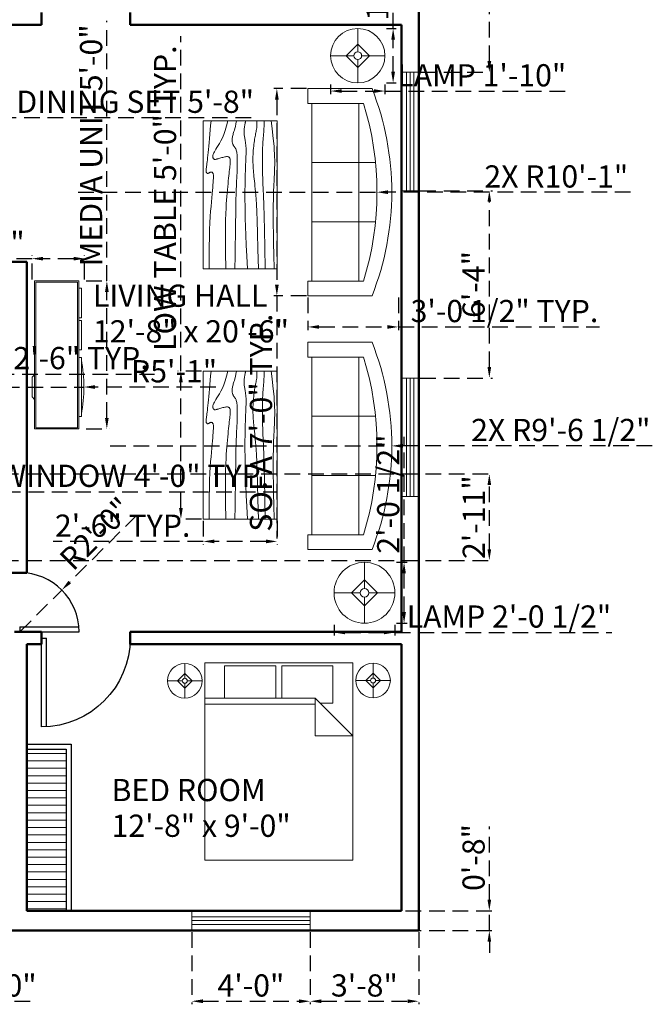
# Model space of a CAD drawing. Units: inches. Extents: x 3209 to 7144, y 1281 to 3076.
# Tile 3 of 5: x 3474 to 3731, y 1281 to 1680. Entities that reach past the tile are written whole.
import ezdxf

# ---------------------------------------------------------------- set-up
doc = ezdxf.new("R2010")
doc.units = ezdxf.units.IN
doc.linetypes.add('HIDDEN', pattern=[9.525, 6.35, -3.175])
for name, color, linetype, lineweight in [('A-ANNO-DIMS', 244, 'HIDDEN', 18), ('A-AREA-IDEN', 7, 'Continuous', 25), ('A-DOOR', 4, 'Continuous', 25), ('A-FLOR-CASE', 8, 'Continuous', 25), ('A-FLOR-CASE-PATT', 252, 'Continuous', 13), ('A-FURN', 8, 'Continuous', 18), ('A-GLAZ', 4, 'Continuous', 18), ('A-WALL', 7, 'Continuous', 50)]:
    doc.layers.add(name, color=color, linetype=linetype, lineweight=lineweight)
doc.styles.get("Standard").update_dxf_attribs({"font": 'arial.ttf'})
doc.dimstyles.new('ISO-25', dxfattribs={"dimtxt": 9, "dimasz": 4.5, "dimexe": 1.25, "dimexo": 0.625, "dimtad": 1, "dimdec": 0, "dimlunit": 3, "dimtxsty": 'Standard', "dimcen": 2.5, "dimadec": 0, "dimazin": 0, "dimtfac": 1, "dimtdec": 0, "dimtmove": 0, "dimatfit": 3, "dimfxl": 1, "dimarcsym": 0})

# ---------------------------------------------------------------- blocks, each defined once
blk = doc.blocks.new('Entertainment Center')
for p, q in [((-4, 0), (-5, -1)), ((4, 0), (-4, 0)), ((5, -1), (4, 0)), ((-17, -19), (-17, -1)), ((-17, -1), (43, -1)), ((-16.5, -18.5), (-16.5, -1.5)), ((-16.5, -1.5), (42.5, -1.5)), ((42.5, -1.5), (42.5, -18.5)), ((43, -1), (43, -19)), ((43, -19), (-17, -19)), ((42.5, -18.5), (-16.5, -18.5)), ((-12, -20), (-12, -19)), ((12, -19), (12, -20)), ((15, -20), (15, -19)), ((27, -19), (27, -20)), ((28, -20), (28, -19)), ((40, -19), (40, -20)), ((12, -20), (-12, -20)), ((27, -20), (15, -20)), ((40, -20), (28, -20))]:
    blk.add_line(p, q)
blk.add_arc((0, 40), 61, 259.6111, 280.3889)
blk = doc.blocks.new('Sofa - Roundback 7 ft.')
for p, q in [((-12.00002, -32.4421), (-12.00003, -6.5971)), ((11.99997, -32.4421), (11.99998, -6.5971)), ((-36.000027, -34), (-36.000027, -11.4696)), ((35.99998, -34), (35.99998, -11.4696)), ((-35.999844, -13.3819), (35.9998, -13.3819)), ((-36.000027, -32.4421), (35.99998, -32.4421))]:
    blk.add_line(p, q)
for points in [[(-36.000027, -34), (-42.000027, -34), (-42.000027, -8)], [(41.99998, -8), (41.99998, -34), (35.99998, -34)]]:
    blk.add_lwpolyline(points)
for centre, radius, start, end in [((0, -114.25), 114.25, 68.43141, 111.5686), ((-0.00001, -127.1968), 121.1968, 72.72033, 107.2797)]:
    blk.add_arc(centre, radius, start, end)
blk = doc.blocks.new('Table - Rectangular Woodgrain 60 x 30 in.')
for p, q in [((0, 0), (0, -30)), ((60, 0), (0, 0)), ((60, -30), (60, 0)), ((0, -30), (60, -30))]:
    blk.add_line(p, q)
for points in [[(0, -2.4), (4.8155, -2.418), (9.0302, -2.4688), (12.709, -2.5477), (15.9167, -2.65), (18.7181, -2.7711), (21.1781, -2.9063), (23.3616, -3.0508), (25.3333, -3.2), (27.1477, -3.3495), (28.8172, -3.4958), (30.3437, -3.636), (31.7291, -3.7667), (32.9756, -3.8849), (34.0849, -3.9875), (35.059, -4.0714), (35.9, -4.1334), (36.6114, -4.1711), (37.2041, -4.1854), (37.6906, -4.1779), (38.0833, -4.15), (38.3948, -4.1034), (38.6375, -4.0396), (38.8239, -3.9602), (38.9666, -3.8667), (39.0764, -3.7608), (39.1573, -3.6448), (39.2116, -3.521), (39.2416, -3.3917), (39.2498, -3.2593), (39.2385, -3.1261), (39.21, -2.9944), (39.1666, -2.8667), (39.111, -2.7447), (39.0468, -2.6281), (38.978, -2.5163), (38.9083, -2.4083), (38.8418, -2.3035), (38.7823, -2.201), (38.7337, -2.1001), (38.7, -2), (38.6844, -1.9003), (38.6875, -1.8021), (38.7094, -1.707), (38.75, -1.6167), (38.8094, -1.5326), (38.8875, -1.4563), (38.9844, -1.3893), (39.1, -1.3333), (39.2351, -1.2896), (39.3937, -1.2583), (39.5804, -1.2396), (39.8, -1.2333), (40.057, -1.2396), (40.3562, -1.2583), (40.7023, -1.2896), (41.1, -1.3333), (41.5547, -1.3895), (42.0755, -1.4573), (42.6721, -1.5361), (43.3542, -1.625), (44.1316, -1.7233), (45.014, -1.8302), (46.0114, -1.9449), (47.1333, -2.0667), (48.3862, -2.1947), (49.7625, -2.3281), (51.2513, -2.4663), (52.8416, -2.6083), (54.5226, -2.7535), (56.2833, -2.9011), (58.1127, -3.0501), (60, -3.2)], [(0, -9.2), (6.5759, -9.0858), (11.9385, -9.0365), (16.2527, -9.0418), (19.6833, -9.0917), (22.3952, -9.1759), (24.5531, -9.2844), (26.322, -9.4069), (27.8666, -9.5333), (29.3241, -9.6553), (30.7203, -9.7719), (32.0532, -9.8837), (33.3208, -9.9917), (34.5213, -10.0965), (35.6526, -10.199), (36.7128, -10.2999), (37.7, -10.4), (38.6129, -10.4996), (39.4531, -10.5969), (40.223, -10.6895), (40.925, -10.775), (41.5613, -10.8512), (42.1344, -10.9156), (42.6465, -10.966), (43.1, -11), (43.4976, -11.0158), (43.8437, -11.0136), (44.143, -10.9942), (44.4, -10.9583), (44.6195, -10.9069), (44.8062, -10.8406), (44.9648, -10.7603), (45.1, -10.6667), (45.2155, -10.5598), (45.3114, -10.4365), (45.3871, -10.2929), (45.4416, -10.125), (45.4743, -9.929), (45.4844, -9.7011), (45.4709, -9.4371), (45.4333, -9.1333), (45.3716, -8.7883), (45.2896, -8.4104), (45.1919, -8.0107), (45.0833, -7.6), (44.9685, -7.1893), (44.8521, -6.7896), (44.7388, -6.4117), (44.6333, -6.0667), (44.54, -5.7628), (44.4614, -5.4979), (44.4001, -5.2675), (44.3583, -5.0667), (44.3384, -4.8909), (44.3427, -4.7354), (44.3736, -4.5956), (44.4333, -4.4667), (44.5236, -4.3453), (44.6427, -4.2333), (44.7884, -4.1339), (44.9583, -4.05), (45.1501, -3.9849), (45.3614, -3.9417), (45.59, -3.9234), (45.8333, -3.9333), (46.0915, -3.9749), (46.3734, -4.0531), (46.6906, -4.1736), (47.0542, -4.3417), (47.4756, -4.5629), (47.9661, -4.8427), (48.5372, -5.1866), (49.2, -5.6), (49.9676, -6.0844), (50.8594, -6.625), (51.8965, -7.2031), (53.1, -7.8), (54.491, -8.3969), (56.0906, -8.975), (57.9199, -9.5156), (60, -10)], [(0, -12.8), (5.1847, -12.9322), (9.6213, -13.0323), (13.3963, -13.1059), (16.5958, -13.1583), (19.3063, -13.1952), (21.614, -13.2219), (23.6054, -13.2439), (25.3666, -13.2667), (26.9728, -13.2947), (28.4531, -13.3281), (29.8256, -13.3663), (31.1083, -13.4083), (32.3191, -13.4535), (33.476, -13.501), (34.597, -13.5501), (35.7, -13.6), (36.7984, -13.6497), (37.8875, -13.6979), (38.9578, -13.743), (40, -13.7833), (41.0047, -13.8174), (41.9625, -13.8438), (42.864, -13.8607), (43.7, -13.8667), (44.4631, -13.8604), (45.1552, -13.8417), (45.7801, -13.8104), (46.3416, -13.7667), (46.8439, -13.7104), (47.2906, -13.6417), (47.6858, -13.5604), (48.0333, -13.4667), (48.3375, -13.3608), (48.6042, -13.2448), (48.8396, -13.121), (49.05, -12.9917), (49.2417, -12.8593), (49.4208, -12.7261), (49.5937, -12.5944), (49.7667, -12.4667), (49.9452, -12.3451), (50.1323, -12.2313), (50.3303, -12.1268), (50.5416, -12.0333), (50.7686, -11.9524), (51.0135, -11.8854), (51.2788, -11.8341), (51.5666, -11.8), (51.8785, -11.7843), (52.2116, -11.7865), (52.562, -11.8059), (52.926, -11.8417), (53.2998, -11.8931), (53.6795, -11.9594), (54.0614, -12.0397), (54.4416, -12.1333), (54.8223, -12.2401), (55.2293, -12.3625), (55.6942, -12.5037), (56.2489, -12.6667), (56.9251, -12.8547), (57.7545, -13.0708), (58.7689, -13.3182), (60, -13.6)], [(0, -18), (5.124, -17.7273), (9.6609, -17.5057), (13.6705, -17.3303), (17.2125, -17.1958), (20.3467, -17.0973), (23.1328, -17.0297), (25.6307, -16.9878), (27.9, -16.9667), (29.9928, -16.9617), (31.9302, -16.9703), (33.7254, -16.9907), (35.3917, -17.0208), (36.9423, -17.0588), (38.3906, -17.1026), (39.7499, -17.1503), (41.0333, -17.2), (42.2519, -17.2496), (43.4073, -17.2969), (44.4986, -17.3395), (45.525, -17.375), (46.4858, -17.4012), (47.3802, -17.4156), (48.2074, -17.416), (48.9667, -17.4), (49.6583, -17.3662), (50.2872, -17.3167), (50.8595, -17.2547), (51.3812, -17.1833), (51.8584, -17.1057), (52.2971, -17.025), (52.7034, -16.9443), (53.0833, -16.8667), (53.443, -16.7951), (53.789, -16.7313), (54.128, -16.6768), (54.4666, -16.6334), (54.8115, -16.6024), (55.1693, -16.5854), (55.5465, -16.5841), (55.95, -16.6), (56.3828, -16.6337), (56.8346, -16.6823), (57.2915, -16.7418), (57.7396, -16.8084), (58.165, -16.878), (58.5539, -16.9469), (58.8924, -17.0111), (59.1666, -17.0667), (59.3679, -17.1107), (59.5078, -17.1438), (59.6032, -17.1675), (59.6708, -17.1833), (59.7275, -17.193), (59.7901, -17.1979), (59.8753, -17.1998), (60, -17.2)], [(0, -22.4), (8.0098, -22.2501), (14.4094, -22.1011), (19.4168, -21.9535), (23.25, -21.8083), (26.1269, -21.6663), (28.2656, -21.5281), (29.884, -21.3947), (31.2, -21.2667), (32.3967, -21.1448), (33.5172, -21.0292), (34.5697, -20.9198), (35.5625, -20.8167), (36.5037, -20.7198), (37.4015, -20.6292), (38.2642, -20.5448), (39.1, -20.4667), (39.9164, -20.3951), (40.7187, -20.3313), (41.5117, -20.2768), (42.3, -20.2333), (43.0883, -20.2024), (43.8812, -20.1854), (44.6836, -20.1841), (45.5, -20.2), (46.3328, -20.234), (47.1747, -20.2844), (48.0163, -20.3488), (48.8479, -20.425), (49.66, -20.5106), (50.4429, -20.6031), (51.1872, -20.7004), (51.8833, -20.8), (52.5246, -20.8999), (53.1166, -20.9995), (53.6681, -21.0983), (54.1875, -21.1958), (54.6834, -21.2919), (55.1646, -21.3859), (55.6394, -21.4777), (56.1167, -21.5667), (56.6028, -21.6515), (57.0961, -21.7266), (57.5929, -21.7852), (58.0896, -21.8208), (58.5823, -21.8268), (59.0674, -21.7964), (59.5412, -21.723), (60, -21.6)], [(0, -25.2), (8.6355, -25.0504), (15.7026, -24.9031), (21.4049, -24.7606), (25.9458, -24.625), (29.529, -24.4988), (32.3578, -24.3844), (34.6359, -24.284), (36.5667, -24.2), (38.3213, -24.1341), (39.9417, -24.0854), (41.437, -24.0523), (42.8167, -24.0333), (44.0901, -24.0268), (45.2667, -24.0313), (46.3557, -24.0451), (47.3667, -24.0667), (48.309, -24.0947), (49.1928, -24.1287), (50.0284, -24.168), (50.826, -24.2125), (51.5959, -24.2617), (52.3483, -24.3151), (53.0935, -24.3725), (53.8417, -24.4334), (54.6009, -24.497), (55.3699, -24.561), (56.1454, -24.6226), (56.9239, -24.6792), (57.7021, -24.7279), (58.4764, -24.7662), (59.2435, -24.7911), (60, -24.8)], [(0, -28.8), (5.6867, -28.6681), (10.45, -28.5698), (14.407, -28.5012), (17.675, -28.4584), (20.3711, -28.4374), (22.6125, -28.4344), (24.5164, -28.4455), (26.2, -28.4667), (27.762, -28.4947), (29.2276, -28.5281), (30.6033, -28.5663), (31.8958, -28.6084), (33.1118, -28.6535), (34.2578, -28.7011), (35.3405, -28.7501), (36.3666, -28.8), (37.3443, -28.8497), (38.288, -28.8974), (39.2137, -28.9412), (40.1375, -28.9792), (41.0753, -29.0093), (42.0432, -29.0297), (43.0572, -29.0384), (44.1333, -29.0333), (45.2936, -29.0114), (46.5843, -28.9641), (48.0579, -28.8816), (49.7666, -28.7542), (51.7629, -28.5721), (54.0989, -28.3255), (56.8272, -28.0048), (60, -27.6)]]:
    blk.add_lwpolyline(points)
blk = doc.blocks.new('Bed - Queen')
for p, q in [((0, -80.00003), (0, 0)), ((0, 0), (59.99999, 0)), ((59.99999, 0), (59.99999, -80.00003)), ((7.99999, -1.2), (28.79998, -1.2)), ((7.99999, -14.4), (7.99999, -1.2)), ((28.79998, -1.2), (28.79998, -14.4)), ((31.19999, -1.2), (51.99999, -1.2)), ((31.19999, -14.4), (31.19999, -1.2)), ((51.99999, -1.2), (51.99999, -16.4)), ((0, -14.4), (44.8, -14.4)), ((59.99999, -29.6), (44.8, -14.4)), ((44.8, -14.4), (44.8, -29.6)), ((44.8, -16.8), (0, -16.8)), ((51.99999, -16.4), (46.79936, -16.4)), ((44.8, -29.6), (59.99999, -29.6)), ((59.99999, -80.00003), (0, -80.00003))]:
    blk.add_line(p, q)
blk = doc.blocks.new('Lamp - Table')
for p, q in [((0, 7), (0, 1)), ((0, 3), (-3, 0)), ((3, 0), (0, 3)), ((-1, 0), (-7, 0)), ((-3, 0), (0, -3)), ((0, -3), (3, 0)), ((1, 0), (7, 0)), ((0, -1), (0, -7))]:
    blk.add_line(p, q)
for radius in [7, 1]:
    blk.add_circle((0, 0), radius)
blk = doc.blocks.new('DOOR-SWING-36IN')
for p, q in [((0, 36), (0, 0)), ((2, 36), (2, 0)), ((0, 0), (2, 0))]:
    blk.add_line(p, q)
blk.add_arc((0, 0), 36, 0, 90)
blk = doc.blocks.new('WINDOW-48IN-WALL7')
for p, q in [((0, 48), (7, 48)), ((2, 48), (2, 0)), ((3.5, 48), (3.5, 0)), ((5, 48), (5, 0)), ((0, 0), (7, 0))]:
    blk.add_line(p, q)
blk = doc.blocks.new('CASEWORK-BEDROOM-SURROUND')
for p, q in [((0, 67.48), (18, 67.48)), ((0, 65.48), (16, 65.48)), ((16, 65.48), (16, 0)), ((18, 67.48), (18, 0))]:
    blk.add_line(p, q)
blk = doc.blocks.new('*D26')
at = {"layer": 'A-ANNO-DIMS', "color": 0, "lineweight": -2, "transparency": 16777216}
for p, q in [((3600.19, 1654.1), (3600.19, 1650.17)), ((3622.25, 1654.1), (3622.25, 1650.17)), ((3604.69, 1651.42), (3617.75, 1651.42)), ((3622.25, 1651.42), (3696.25, 1651.42))]:
    blk.add_line(p, q, dxfattribs=at)
at = {"layer": 'A-ANNO-DIMS', "color": 0, "transparency": 16777216}
for points in [[(3604.69, 1652.17), (3604.69, 1650.67), (3600.19, 1651.42)], [(3617.75, 1652.17), (3617.75, 1650.67), (3622.25, 1651.42)]]:
    blk.add_solid(points, dxfattribs=at)
at = {"layer": 'Defpoints', "color": 0, "transparency": 16777216}
for p in [(3600.19, 1654.72), (3622.25, 1654.72), (3622.25, 1651.42)]:
    blk.add_point(p, dxfattribs=at)
at = {"layer": 'A-ANNO-DIMS', "color": 0, "transparency": 16777216, "insert": (3661.5, 1656.64), "char_height": 9, "attachment_point": 5}
blk.add_mtext('LAMP 1\'-10"', dxfattribs=at)
blk = doc.blocks.new('*D27')
at = {"layer": 'A-ANNO-DIMS', "color": 0, "lineweight": -2, "transparency": 16777216}
for p, q in [((3625.56, 1676.78), (3625.56, 1712.6)), ((3622.87, 1676.78), (3626.81, 1676.78)), ((3625.56, 1659.22), (3625.56, 1672.28)), ((3622.87, 1654.72), (3626.81, 1654.72))]:
    blk.add_line(p, q, dxfattribs=at)
at = {"layer": 'A-ANNO-DIMS', "color": 0, "transparency": 16777216}
for points in [[(3624.81, 1672.28), (3626.31, 1672.28), (3625.56, 1676.78)], [(3624.81, 1659.22), (3626.31, 1659.22), (3625.56, 1654.72)]]:
    blk.add_solid(points, dxfattribs=at)
at = {"layer": 'Defpoints', "color": 0, "transparency": 16777216}
for p in [(3622.25, 1676.78), (3625.56, 1676.78), (3622.25, 1654.72)]:
    blk.add_point(p, dxfattribs=at)
at = {"layer": 'A-ANNO-DIMS', "color": 0, "transparency": 16777216, "insert": (3620.34, 1696.94), "char_height": 9, "attachment_point": 5, "rotation": 90}
blk.add_mtext('1\'-10"', dxfattribs=at)
blk = doc.blocks.new('*D28')
at = {"layer": 'A-ANNO-DIMS', "color": 0, "lineweight": -2, "transparency": 16777216}
for p, q in [((3601.6, 1435.14), (3601.6, 1430.81)), ((3626.3, 1435.14), (3626.3, 1430.81)), ((3606.1, 1432.06), (3621.8, 1432.06)), ((3626.3, 1432.06), (3714.28, 1432.06))]:
    blk.add_line(p, q, dxfattribs=at)
at = {"layer": 'A-ANNO-DIMS', "color": 0, "transparency": 16777216}
for points in [[(3606.1, 1432.81), (3606.1, 1431.31), (3601.6, 1432.06)], [(3621.8, 1432.81), (3621.8, 1431.31), (3626.3, 1432.06)]]:
    blk.add_solid(points, dxfattribs=at)
at = {"layer": 'Defpoints', "color": 0, "transparency": 16777216}
for p in [(3601.6, 1435.77), (3626.3, 1435.77), (3626.3, 1432.06)]:
    blk.add_point(p, dxfattribs=at)
at = {"layer": 'A-ANNO-DIMS', "color": 0, "transparency": 16777216, "insert": (3672.54, 1437.34), "char_height": 9, "attachment_point": 5}
blk.add_mtext('LAMP 2\'-0 1/2"', dxfattribs=at)
blk = doc.blocks.new('*D29')
at = {"layer": 'A-ANNO-DIMS', "color": 0, "lineweight": -2, "transparency": 16777216}
for p, q in [((3630, 1460.47), (3630, 1511.27)), ((3626.93, 1460.47), (3631.25, 1460.47)), ((3630, 1440.27), (3630, 1455.97)), ((3626.93, 1435.77), (3631.25, 1435.77))]:
    blk.add_line(p, q, dxfattribs=at)
at = {"layer": 'A-ANNO-DIMS', "color": 0, "transparency": 16777216}
for points in [[(3629.25, 1455.97), (3630.75, 1455.97), (3630, 1460.47)], [(3629.25, 1440.27), (3630.75, 1440.27), (3630, 1435.77)]]:
    blk.add_solid(points, dxfattribs=at)
at = {"layer": 'Defpoints', "color": 0, "transparency": 16777216}
for p in [(3626.3, 1460.47), (3630, 1460.47), (3626.3, 1435.77)]:
    blk.add_point(p, dxfattribs=at)
at = {"layer": 'A-ANNO-DIMS', "color": 0, "transparency": 16777216, "insert": (3624.73, 1488.12), "char_height": 9, "attachment_point": 5, "rotation": 90}
blk.add_mtext('2\'-0 1/2"', dxfattribs=at)
blk = doc.blocks.new('*D34')
at = {"layer": 'A-ANNO-DIMS', "color": 0, "lineweight": -2, "transparency": 16777216}
for p, q in [((3539.5, 1537.94), (3539.5, 1673.6)), ((3547.87, 1537.94), (3538.25, 1537.94)), ((3539.5, 1482.44), (3539.5, 1533.44)), ((3547.87, 1477.94), (3538.25, 1477.94))]:
    blk.add_line(p, q, dxfattribs=at)
at = {"layer": 'A-ANNO-DIMS', "color": 0, "transparency": 16777216}
for points in [[(3538.75, 1533.44), (3540.25, 1533.44), (3539.5, 1537.94)], [(3538.75, 1482.44), (3540.25, 1482.44), (3539.5, 1477.94)]]:
    blk.add_solid(points, dxfattribs=at)
at = {"layer": 'Defpoints', "color": 0, "transparency": 16777216}
for p in [(3539.5, 1537.94), (3548.5, 1537.94), (3548.5, 1477.94)]:
    blk.add_point(p, dxfattribs=at)
at = {"layer": 'A-ANNO-DIMS', "color": 0, "transparency": 16777216, "insert": (3534.22, 1608.02), "char_height": 9, "attachment_point": 5, "rotation": 90}
blk.add_mtext('LOW TABLE 5\'-0" TYP.', dxfattribs=at)
blk = doc.blocks.new('*D35')
at = {"layer": 'A-ANNO-DIMS', "color": 0, "lineweight": -2, "transparency": 16777216}
for p, q in [((3548.5, 1477.31), (3548.5, 1467.69)), ((3578.5, 1477.31), (3578.5, 1467.69)), ((3548.5, 1468.94), (3487.74, 1468.94)), ((3574, 1468.94), (3553, 1468.94))]:
    blk.add_line(p, q, dxfattribs=at)
at = {"layer": 'A-ANNO-DIMS', "color": 0, "transparency": 16777216}
for points in [[(3553, 1469.69), (3553, 1468.19), (3548.5, 1468.94)], [(3574, 1469.69), (3574, 1468.19), (3578.5, 1468.94)]]:
    blk.add_solid(points, dxfattribs=at)
at = {"layer": 'Defpoints', "color": 0, "transparency": 16777216}
for p in [(3548.5, 1477.94), (3578.5, 1477.94), (3548.5, 1468.94)]:
    blk.add_point(p, dxfattribs=at)
at = {"layer": 'A-ANNO-DIMS', "color": 0, "transparency": 16777216, "insert": (3515.87, 1474.16), "char_height": 9, "attachment_point": 5}
blk.add_mtext('2\'-6" TYP.', dxfattribs=at)
blk = doc.blocks.new('*D40')
at = {"layer": 'A-ANNO-DIMS', "color": 0, "lineweight": -2, "transparency": 16777216}
for p, q in [((3590.38, 1652.44), (3577.16, 1652.44)), ((3578.41, 1647.94), (3578.41, 1572.94)), ((3590.38, 1568.44), (3577.16, 1568.44)), ((3578.41, 1568.44), (3578.41, 1470.15))]:
    blk.add_line(p, q, dxfattribs=at)
at = {"layer": 'A-ANNO-DIMS', "color": 0, "transparency": 16777216}
for points in [[(3577.66, 1647.94), (3579.16, 1647.94), (3578.41, 1652.44)], [(3577.66, 1572.94), (3579.16, 1572.94), (3578.41, 1568.44)]]:
    blk.add_solid(points, dxfattribs=at)
at = {"layer": 'Defpoints', "color": 0, "transparency": 16777216}
for p in [(3591.01, 1652.44), (3578.41, 1568.44), (3591.01, 1568.44)]:
    blk.add_point(p, dxfattribs=at)
at = {"layer": 'A-ANNO-DIMS', "color": 0, "transparency": 16777216, "insert": (3573.13, 1517.05), "char_height": 9, "attachment_point": 5, "rotation": 90}
blk.add_mtext('SOFA 7\'-0" TYP.', dxfattribs=at)
blk = doc.blocks.new('*D41')
at = {"layer": 'A-ANNO-DIMS', "color": 0, "lineweight": -2, "transparency": 16777216}
for p, q in [((3591.01, 1567.82), (3591.01, 1554.59)), ((3627.68, 1567.82), (3627.68, 1554.59)), ((3595.51, 1555.84), (3623.18, 1555.84)), ((3627.68, 1555.84), (3709.25, 1555.84))]:
    blk.add_line(p, q, dxfattribs=at)
at = {"layer": 'A-ANNO-DIMS', "color": 0, "transparency": 16777216}
for points in [[(3595.51, 1556.59), (3595.51, 1555.09), (3591.01, 1555.84)], [(3623.18, 1556.59), (3623.18, 1555.09), (3627.68, 1555.84)]]:
    blk.add_solid(points, dxfattribs=at)
at = {"layer": 'Defpoints', "color": 0, "transparency": 16777216}
for p in [(3591.01, 1568.44), (3627.68, 1568.44), (3627.68, 1555.84)]:
    blk.add_point(p, dxfattribs=at)
at = {"layer": 'A-ANNO-DIMS', "color": 0, "transparency": 16777216, "insert": (3670.71, 1561.12), "char_height": 9, "attachment_point": 5}
blk.add_mtext('3\'-0 1/2" TYP.', dxfattribs=at)
blk = doc.blocks.new('*D42')
at = {"layer": 'A-ANNO-DIMS', "color": 0, "lineweight": -2, "transparency": 16777216}
for p, q in [((3397.44, 1540.64), (3397.44, 1535.52)), ((3427.44, 1540.64), (3427.44, 1535.52)), ((3401.94, 1536.77), (3422.94, 1536.77)), ((3427.44, 1536.77), (3528.81, 1536.77))]:
    blk.add_line(p, q, dxfattribs=at)
at = {"layer": 'A-ANNO-DIMS', "color": 0, "transparency": 16777216}
for points in [[(3401.94, 1537.52), (3401.94, 1536.02), (3397.44, 1536.77)], [(3422.94, 1537.52), (3422.94, 1536.02), (3427.44, 1536.77)]]:
    blk.add_solid(points, dxfattribs=at)
at = {"layer": 'Defpoints', "color": 0, "transparency": 16777216}
for p in [(3397.44, 1541.27), (3427.44, 1541.27), (3427.44, 1536.77)]:
    blk.add_point(p, dxfattribs=at)
at = {"layer": 'A-ANNO-DIMS', "color": 0, "transparency": 16777216, "insert": (3480.37, 1542.05), "char_height": 9, "attachment_point": 5}
blk.add_mtext('DOOR 2\'-6" TYP.', dxfattribs=at)
blk = doc.blocks.new('*D46')
at = {"layer": 'A-ANNO-DIMS', "color": 0, "lineweight": -2, "transparency": 16777216}
for p, q in [((3410.58, 1495.64), (3410.58, 1487.82)), ((3458.58, 1495.64), (3458.58, 1487.82)), ((3415.08, 1489.07), (3454.08, 1489.07)), ((3458.58, 1489.07), (3578.22, 1489.07))]:
    blk.add_line(p, q, dxfattribs=at)
at = {"layer": 'A-ANNO-DIMS', "color": 0, "transparency": 16777216}
for points in [[(3415.08, 1489.82), (3415.08, 1488.32), (3410.58, 1489.07)], [(3454.08, 1489.82), (3454.08, 1488.32), (3458.58, 1489.07)]]:
    blk.add_solid(points, dxfattribs=at)
at = {"layer": 'Defpoints', "color": 0, "transparency": 16777216}
for p in [(3410.58, 1496.27), (3458.58, 1496.27), (3458.58, 1489.07)]:
    blk.add_point(p, dxfattribs=at)
at = {"layer": 'A-ANNO-DIMS', "color": 0, "transparency": 16777216, "insert": (3520.65, 1494.35), "char_height": 9, "attachment_point": 5}
blk.add_mtext('WINDOW 4\'-0" TYP.', dxfattribs=at)
blk = doc.blocks.new('*D52')
at = {"layer": 'A-ANNO-DIMS', "color": 0, "lineweight": -2, "transparency": 16777216}
for p, q in [((3398.32, 1631.06), (3398.32, 1641.9)), ((3402.82, 1640.65), (3461.88, 1640.65)), ((3466.38, 1631.06), (3466.38, 1641.9)), ((3466.38, 1640.65), (3571.05, 1640.65))]:
    blk.add_line(p, q, dxfattribs=at)
at = {"layer": 'A-ANNO-DIMS', "color": 0, "transparency": 16777216}
for points in [[(3402.82, 1641.4), (3402.82, 1639.9), (3398.32, 1640.65)], [(3461.88, 1641.4), (3461.88, 1639.9), (3466.38, 1640.65)]]:
    blk.add_solid(points, dxfattribs=at)
at = {"layer": 'Defpoints', "color": 0, "transparency": 16777216}
for p in [(3466.38, 1640.65), (3398.32, 1630.44), (3466.38, 1630.44)]:
    blk.add_point(p, dxfattribs=at)
at = {"layer": 'A-ANNO-DIMS', "color": 0, "transparency": 16777216, "insert": (3520.96, 1645.92), "char_height": 9, "attachment_point": 5}
blk.add_mtext('DINING SET 5\'-8"', dxfattribs=at)
blk = doc.blocks.new('*D54')
at = {"layer": 'A-ANNO-DIMS', "color": 0, "lineweight": -2, "transparency": 16777216}
for p, q in [((3509.46, 1574.5), (3509.46, 1679.9)), ((3501.08, 1574.5), (3510.71, 1574.5)), ((3509.46, 1519), (3509.46, 1570)), ((3501.08, 1514.5), (3510.71, 1514.5))]:
    blk.add_line(p, q, dxfattribs=at)
at = {"layer": 'A-ANNO-DIMS', "color": 0, "transparency": 16777216}
for points in [[(3508.71, 1570), (3510.21, 1570), (3509.46, 1574.5)], [(3508.71, 1519), (3510.21, 1519), (3509.46, 1514.5)]]:
    blk.add_solid(points, dxfattribs=at)
at = {"layer": 'Defpoints', "color": 0, "transparency": 16777216}
for p in [(3500.46, 1574.5), (3509.46, 1574.5), (3500.46, 1514.5)]:
    blk.add_point(p, dxfattribs=at)
at = {"layer": 'A-ANNO-DIMS', "color": 0, "transparency": 16777216, "insert": (3504.24, 1629.45), "char_height": 9, "attachment_point": 5, "rotation": 90}
blk.add_mtext('MEDIA UNIT 5\'-0"', dxfattribs=at)
blk = doc.blocks.new('*D55')
at = {"layer": 'A-ANNO-DIMS', "color": 0, "lineweight": -2, "transparency": 16777216}
for p, q in [((3479.12, 1575.13), (3479.12, 1584.75)), ((3500.46, 1575.13), (3500.46, 1584.75)), ((3479.12, 1583.5), (3429.33, 1583.5)), ((3495.96, 1583.5), (3483.62, 1583.5))]:
    blk.add_line(p, q, dxfattribs=at)
at = {"layer": 'A-ANNO-DIMS', "color": 0, "transparency": 16777216}
for points in [[(3483.62, 1584.25), (3483.62, 1582.75), (3479.12, 1583.5)], [(3495.96, 1584.25), (3495.96, 1582.75), (3500.46, 1583.5)]]:
    blk.add_solid(points, dxfattribs=at)
at = {"layer": 'Defpoints', "color": 0, "transparency": 16777216}
for p in [(3479.12, 1583.5), (3479.12, 1574.5), (3500.46, 1574.5)]:
    blk.add_point(p, dxfattribs=at)
at = {"layer": 'A-ANNO-DIMS', "color": 0, "transparency": 16777216, "insert": (3451.97, 1588.78), "char_height": 9, "attachment_point": 5}
blk.add_mtext('1\'-9 1/2"', dxfattribs=at)
blk = doc.blocks.new('*D66')
at = {"layer": 'A-ANNO-DIMS', "color": 0, "lineweight": -2, "transparency": 16777216}
for p, q in [((3543.89, 1310.64), (3543.89, 1281.37)), ((3591.89, 1310.64), (3591.89, 1281.37)), ((3548.39, 1282.62), (3587.39, 1282.62))]:
    blk.add_line(p, q, dxfattribs=at)
at = {"layer": 'A-ANNO-DIMS', "color": 0, "transparency": 16777216}
for points in [[(3548.39, 1283.37), (3548.39, 1281.87), (3543.89, 1282.62)], [(3587.39, 1283.37), (3587.39, 1281.87), (3591.89, 1282.62)]]:
    blk.add_solid(points, dxfattribs=at)
at = {"layer": 'Defpoints', "color": 0, "transparency": 16777216}
for p in [(3543.89, 1311.27), (3591.89, 1311.27), (3591.89, 1282.62)]:
    blk.add_point(p, dxfattribs=at)
at = {"layer": 'A-ANNO-DIMS', "color": 0, "transparency": 16777216, "insert": (3567.89, 1287.85), "char_height": 9, "attachment_point": 5}
blk.add_mtext('4\'-0"', dxfattribs=at)
blk = doc.blocks.new('*D67')
at = {"layer": 'A-ANNO-DIMS', "color": 0, "lineweight": -2, "transparency": 16777216}
for p, q in [((3591.89, 1310.64), (3591.89, 1281.37)), ((3635.94, 1310.64), (3635.94, 1281.37)), ((3596.39, 1282.62), (3631.44, 1282.62))]:
    blk.add_line(p, q, dxfattribs=at)
at = {"layer": 'A-ANNO-DIMS', "color": 0, "transparency": 16777216}
for points in [[(3596.39, 1283.37), (3596.39, 1281.87), (3591.89, 1282.62)], [(3631.44, 1283.37), (3631.44, 1281.87), (3635.94, 1282.62)]]:
    blk.add_solid(points, dxfattribs=at)
at = {"layer": 'Defpoints', "color": 0, "transparency": 16777216}
for p in [(3591.89, 1311.27), (3635.94, 1311.27), (3635.94, 1282.62)]:
    blk.add_point(p, dxfattribs=at)
at = {"layer": 'A-ANNO-DIMS', "color": 0, "transparency": 16777216, "insert": (3613.91, 1287.85), "char_height": 9, "attachment_point": 5}
blk.add_mtext('3\'-8"', dxfattribs=at)
blk = doc.blocks.new('*D68')
at = {"layer": 'A-ANNO-DIMS', "color": 0, "lineweight": -2, "transparency": 16777216}
for p, q in [((3664.58, 1323.77), (3664.58, 1353.44)), ((3592.51, 1319.27), (3665.83, 1319.27)), ((3664.58, 1311.27), (3664.58, 1319.27)), ((3592.51, 1311.27), (3665.83, 1311.27)), ((3664.58, 1306.77), (3664.58, 1302.27))]:
    blk.add_line(p, q, dxfattribs=at)
at = {"layer": 'A-ANNO-DIMS', "color": 0, "transparency": 16777216}
for points in [[(3663.83, 1323.77), (3665.33, 1323.77), (3664.58, 1319.27)], [(3663.83, 1306.77), (3665.33, 1306.77), (3664.58, 1311.27)]]:
    blk.add_solid(points, dxfattribs=at)
at = {"layer": 'Defpoints', "color": 0, "transparency": 16777216}
for p in [(3591.89, 1319.27), (3664.58, 1319.27), (3591.89, 1311.27)]:
    blk.add_point(p, dxfattribs=at)
at = {"layer": 'A-ANNO-DIMS', "color": 0, "transparency": 16777216, "insert": (3659.36, 1340.86), "char_height": 9, "attachment_point": 5, "rotation": 90}
blk.add_mtext('0\'-8"', dxfattribs=at)
blk = doc.blocks.new('*D72')
at = {"layer": 'A-ANNO-DIMS', "color": 0, "lineweight": -2, "transparency": 16777216}
for p, q in [((3428.94, 1419.64), (3428.94, 1281.37)), ((3438.94, 1419.64), (3438.94, 1281.37)), ((3424.44, 1282.62), (3419.94, 1282.62)), ((3428.94, 1282.62), (3438.94, 1282.62)), ((3443.44, 1282.62), (3480.11, 1282.62))]:
    blk.add_line(p, q, dxfattribs=at)
at = {"layer": 'A-ANNO-DIMS', "color": 0, "transparency": 16777216}
for points in [[(3424.44, 1283.37), (3424.44, 1281.87), (3428.94, 1282.62)], [(3443.44, 1283.37), (3443.44, 1281.87), (3438.94, 1282.62)]]:
    blk.add_solid(points, dxfattribs=at)
at = {"layer": 'Defpoints', "color": 0, "transparency": 16777216}
for p in [(3428.94, 1420.27), (3438.94, 1420.27), (3438.94, 1282.62)]:
    blk.add_point(p, dxfattribs=at)
at = {"layer": 'A-ANNO-DIMS', "color": 0, "transparency": 16777216, "insert": (3464.02, 1287.85), "char_height": 9, "attachment_point": 5}
blk.add_mtext('0\'-10"', dxfattribs=at)
blk = doc.blocks.new('*D73')
at = {"layer": 'A-ANNO-DIMS', "color": 0, "lineweight": -2, "transparency": 16777216}
for p, q in [((3400.56, 1496.27), (3665.83, 1496.27)), ((3664.58, 1465.77), (3664.58, 1491.77)), ((3400.56, 1461.27), (3665.83, 1461.27))]:
    blk.add_line(p, q, dxfattribs=at)
at = {"layer": 'A-ANNO-DIMS', "color": 0, "transparency": 16777216}
for points in [[(3663.83, 1491.77), (3665.33, 1491.77), (3664.58, 1496.27)], [(3663.83, 1465.77), (3665.33, 1465.77), (3664.58, 1461.27)]]:
    blk.add_solid(points, dxfattribs=at)
at = {"layer": 'Defpoints', "color": 0, "transparency": 16777216}
for p in [(3399.94, 1496.27), (3664.58, 1496.27), (3399.94, 1461.27)]:
    blk.add_point(p, dxfattribs=at)
at = {"layer": 'A-ANNO-DIMS', "color": 0, "transparency": 16777216, "insert": (3659.44, 1478.77), "char_height": 9, "attachment_point": 5, "rotation": 90}
blk.add_mtext('2\'-11"', dxfattribs=at)
blk = doc.blocks.new('*D79')
at = {"layer": 'A-ANNO-DIMS', "color": 0, "lineweight": -2, "transparency": 16777216}
for p, q in [((3636.56, 1740.13), (3665.83, 1740.13)), ((3664.58, 1663.54), (3664.58, 1735.63)), ((3636.56, 1659.04), (3665.83, 1659.04))]:
    blk.add_line(p, q, dxfattribs=at)
at = {"layer": 'A-ANNO-DIMS', "color": 0, "transparency": 16777216}
for points in [[(3663.83, 1735.63), (3665.33, 1735.63), (3664.58, 1740.13)], [(3663.83, 1663.54), (3665.33, 1663.54), (3664.58, 1659.04)]]:
    blk.add_solid(points, dxfattribs=at)
at = {"layer": 'Defpoints', "color": 0, "transparency": 16777216}
for p in [(3635.94, 1740.13), (3664.58, 1740.13), (3635.94, 1659.04)]:
    blk.add_point(p, dxfattribs=at)
at = {"layer": 'A-ANNO-DIMS', "color": 0, "transparency": 16777216, "insert": (3659.36, 1699.59), "char_height": 9, "attachment_point": 5, "rotation": 90}
blk.add_mtext('6\'-9"', dxfattribs=at)
blk = doc.blocks.new('*D80')
at = {"layer": 'A-ANNO-DIMS', "color": 0, "lineweight": -2, "transparency": 16777216}
for p, q in [((3636.56, 1611.04), (3665.83, 1611.04)), ((3664.58, 1539.59), (3664.58, 1606.54)), ((3636.56, 1535.09), (3665.83, 1535.09))]:
    blk.add_line(p, q, dxfattribs=at)
at = {"layer": 'A-ANNO-DIMS', "color": 0, "transparency": 16777216}
for points in [[(3663.83, 1606.54), (3665.33, 1606.54), (3664.58, 1611.04)], [(3663.83, 1539.59), (3665.33, 1539.59), (3664.58, 1535.09)]]:
    blk.add_solid(points, dxfattribs=at)
at = {"layer": 'Defpoints', "color": 0, "transparency": 16777216}
for p in [(3635.94, 1611.04), (3664.58, 1611.04), (3635.94, 1535.09)]:
    blk.add_point(p, dxfattribs=at)
at = {"layer": 'A-ANNO-DIMS', "color": 0, "transparency": 16777216, "insert": (3659.36, 1573.06), "char_height": 9, "attachment_point": 5, "rotation": 90}
blk.add_mtext('6\'-4"', dxfattribs=at)
blk = doc.blocks.new('*D82')
at = {"layer": 'A-ANNO-DIMS', "color": 0, "lineweight": -2, "transparency": 16777216}
for p, q in [((3521.45, 1479.49), (3494.38, 1452.42)), ((3474.22, 1432.27), (3491.2, 1449.24))]:
    blk.add_line(p, q, dxfattribs=at)
at = {"layer": 'A-ANNO-DIMS', "color": 0, "transparency": 16777216}
blk.add_solid([(3493.85, 1452.95), (3494.91, 1451.89), (3491.2, 1449.24)], dxfattribs=at)
at = {"layer": 'Defpoints', "color": 0, "transparency": 16777216}
for p in [(3491.2, 1449.24), (3474.22, 1432.27)]:
    blk.add_point(p, dxfattribs=at)
at = {"layer": 'A-ANNO-DIMS', "color": 0, "transparency": 16777216, "insert": (3505.81, 1471.24), "char_height": 9, "attachment_point": 5, "rotation": 44.999}
blk.add_mtext('R2\'-0"', dxfattribs=at)
blk = doc.blocks.new('*D83')
at = {"layer": 'A-ANNO-DIMS', "color": 0, "lineweight": -2, "transparency": 16777216}
for p, q in [((3439.12, 1531.5), (3500.12, 1531.5)), ((3553.62, 1531.5), (3504.62, 1531.5))]:
    blk.add_line(p, q, dxfattribs=at)
at = {"layer": 'A-ANNO-DIMS', "color": 0, "transparency": 16777216}
blk.add_solid([(3504.62, 1532.25), (3504.62, 1530.75), (3500.12, 1531.5)], dxfattribs=at)
at = {"layer": 'Defpoints', "color": 0, "transparency": 16777216}
for p in [(3439.12, 1531.5), (3500.12, 1531.5)]:
    blk.add_point(p, dxfattribs=at)
at = {"layer": 'A-ANNO-DIMS', "color": 0, "transparency": 16777216, "insert": (3536.72, 1536.72), "char_height": 9, "attachment_point": 5, "rotation": 0.0002}
blk.add_mtext('R5\'-1"', dxfattribs=at)
blk = doc.blocks.new('*D84')
at = {"layer": 'A-ANNO-DIMS', "color": 0, "lineweight": -2, "transparency": 16777216}
for p, q in [((3497.81, 1610.44), (3619.01, 1610.44)), ((3721.86, 1610.44), (3623.51, 1610.44))]:
    blk.add_line(p, q, dxfattribs=at)
at = {"layer": 'A-ANNO-DIMS', "color": 0, "transparency": 16777216}
blk.add_solid([(3623.51, 1611.19), (3623.51, 1609.69), (3619.01, 1610.44)], dxfattribs=at)
at = {"layer": 'Defpoints', "color": 0, "transparency": 16777216}
for p in [(3497.81, 1610.44), (3619.01, 1610.44)]:
    blk.add_point(p, dxfattribs=at)
at = {"layer": 'A-ANNO-DIMS', "color": 0, "transparency": 16777216, "insert": (3691.73, 1615.66), "char_height": 9, "attachment_point": 5, "rotation": 0}
blk.add_mtext('2X R10\'-1"', dxfattribs=at)
blk = doc.blocks.new('*D85')
at = {"layer": 'A-ANNO-DIMS', "color": 0, "lineweight": -2, "transparency": 16777216}
for p, q in [((3510.76, 1507.64), (3625.01, 1507.64)), ((3730.68, 1507.64), (3629.51, 1507.64))]:
    blk.add_line(p, q, dxfattribs=at)
at = {"layer": 'A-ANNO-DIMS', "color": 0, "transparency": 16777216}
blk.add_solid([(3629.51, 1508.39), (3629.51, 1506.89), (3625.01, 1507.64)], dxfattribs=at)
at = {"layer": 'Defpoints', "color": 0, "transparency": 16777216}
for p in [(3510.76, 1507.64), (3625.01, 1507.64)]:
    blk.add_point(p, dxfattribs=at)
at = {"layer": 'A-ANNO-DIMS', "color": 0, "transparency": 16777216, "insert": (3693.56, 1512.92), "char_height": 9, "attachment_point": 5, "rotation": 0.0001}
blk.add_mtext('2X R9\'-6 1/2"', dxfattribs=at)

msp = doc.modelspace()

# ---------------------------------------------------------------- hatches: boundary and pattern name
at = {"layer": 'A-FLOR-CASE-PATT'}
h = msp.add_hatch(dxfattribs=at)
h.set_pattern_fill('ANSI31', color=256, scale=0.944882, angle=-45, style=0)
h.paths.add_polyline_path([(3476.94, 1319.27), (3492.94, 1319.27), (3492.94, 1384.75), (3476.94, 1384.75)])

# ---------------------------------------------------------------- linework, layer by layer
at = {"layer": 'A-DOOR'}
for p, q in [((3474.22, 1434.27), (3474.22, 1432.27)), ((3474.22, 1434.27), (3498.22, 1434.27)), ((3474.22, 1432.27), (3498.22, 1432.27))]:
    msp.add_line(p, q, dxfattribs=at)
msp.add_arc((3474.22, 1432.27), 24, 0, 90, dxfattribs=at)
at = {"layer": 'A-GLAZ'}
for p, q in [((3543.89, 1311.27), (3543.89, 1319.27)), ((3543.89, 1316.77), (3591.89, 1316.77)), ((3591.89, 1311.27), (3591.89, 1319.27)), ((3543.89, 1315.27), (3591.89, 1315.27)), ((3543.89, 1313.77), (3591.89, 1313.77))]:
    msp.add_line(p, q, dxfattribs=at)
at = {"layer": 'A-WALL'}
for p, q in [((3635.94, 1851.27), (3635.94, 1311.27)), ((3482.94, 1683.27), (3482.94, 1678.27)), ((3518.94, 1683.27), (3518.94, 1678.27)), ((3465.94, 1678.27), (3482.94, 1678.27)), ((3518.94, 1678.27), (3628.94, 1678.27)), ((3628.94, 1678.27), (3628.94, 1432.27)), ((3394.94, 1582.27), (3476.94, 1582.27)), ((3476.94, 1582.27), (3476.94, 1456.27)), ((3282.94, 1456.27), (3476.94, 1456.27)), ((3482.94, 1432.27), (3471.94, 1432.27)), ((3482.94, 1432.27), (3482.94, 1427.27)), ((3628.94, 1432.27), (3518.94, 1432.27)), ((3518.94, 1432.27), (3518.94, 1427.27)), ((3476.94, 1427.27), (3476.94, 1319.27)), ((3482.94, 1427.27), (3476.94, 1427.27)), ((3628.94, 1427.27), (3518.94, 1427.27)), ((3628.94, 1427.27), (3628.94, 1319.27)), ((3628.94, 1319.27), (3476.94, 1319.27)), ((3635.94, 1311.27), (3459.94, 1311.27))]:
    msp.add_line(p, q, dxfattribs=at)

# ---------------------------------------------------------------- block references
at = {"layer": 'A-DOOR', "extrusion": (0, 0, -1), "zscale": -1, "rotation": 180}
msp.add_blockref('DOOR-SWING-36IN', (-3482.94, 1429.77), dxfattribs=at)
at = {"layer": 'A-FLOR-CASE'}
msp.add_blockref('CASEWORK-BEDROOM-SURROUND', (3476.94, 1319.27), dxfattribs=at)
at = {"layer": 'A-FURN'}
for p, xscale, yscale, zscale in [((3611.22, 1665.75), 1.575209287395368, 1.575209287395368, 1.575209287395368), ((3613.95, 1448.12), 1.764083543787443, 1.764083543787443, 1.764083543787443)]:
    msp.add_blockref('Lamp - Table', p, dxfattribs=dict(at, xscale=xscale, yscale=yscale, zscale=zscale))
for name, p, rotation in [('Sofa - Roundback 7 ft.', (3625.01, 1610.44), 270), ('Table - Rectangular Woodgrain 60 x 30 in.', (3548.5, 1579.37), 90), ('Entertainment Center', (3479.12, 1531.5), 90), ('Sofa - Roundback 7 ft.', (3625.01, 1507.64), 270), ('Table - Rectangular Woodgrain 60 x 30 in.', (3548.5, 1477.94), 90)]:
    msp.add_blockref(name, p, dxfattribs=dict(at, rotation=rotation))
for name, p in [('Lamp - Table', (3541.06, 1412.46)), ('Bed - Queen', (3549.16, 1419.78)), ('Lamp - Table', (3617.43, 1412.59))]:
    msp.add_blockref(name, p, dxfattribs=at)
at = {"layer": 'A-GLAZ'}
for p in [(3628.94, 1611.04), (3628.94, 1487.09)]:
    msp.add_blockref('WINDOW-48IN-WALL7', p, dxfattribs=at)

# ---------------------------------------------------------------- texts
at = {"layer": 'A-AREA-IDEN'}
for s, p in [('LIVING HALL', (3503.83, 1564.01)), ('12\'-8" x 20\'-6"', (3503.83, 1549.56)), ('BED ROOM ', (3511.35, 1363.69)), ('12\'-8" x 9\'-0"', (3511.35, 1349.23))]:
    msp.add_text(s, height=9, dxfattribs=at).set_placement(p)

# ---------------------------------------------------------------- dimensions: what is measured, and where the dimension line sits
at = {"layer": 'A-ANNO-DIMS'}
for base, p1, p2, angle, picture, middle in [((3664.58, 1740.13), (3635.94, 1659.04), (3635.94, 1740.13), 90, '*D79', (3659.36, 1699.59)), ((3625.56, 1676.78), (3622.25, 1654.72), (3622.25, 1676.78), 90, '*D27', (3620.34, 1696.94)), ((3664.5832, 1611.0403), (3635.9382, 1535.0855), (3635.9382, 1611.0403), 90, '*D80', (3659.3631, 1573.0629)), ((3479.12, 1583.5), (3500.46, 1574.5), (3479.12, 1574.5), 180, '*D55', (3451.97, 1588.78)), ((3630, 1460.47), (3626.3, 1435.77), (3626.3, 1460.47), 90, '*D29', (3624.73, 1488.12)), ((3664.58, 1496.27), (3399.94, 1461.27), (3399.94, 1496.27), 90, '*D73', (3659.44, 1478.77)), ((3664.58, 1319.27), (3591.89, 1311.27), (3591.89, 1319.27), 90, '*D68', (3659.36, 1340.86))]:
    dim = msp.add_linear_dim(base=base, p1=p1, p2=p2, angle=angle, dimstyle='ISO-25', override={"dimdec": 1, "dimlfac": 1, "dimrnd": 0, "dimzin": 1, "dimdsep": 46, "dimlunit": 4, "dimfrac": 2}, dxfattribs=at)
    dim.commit()
    dim.dimension.update_dxf_attribs({"geometry": picture, "text_midpoint": middle})
for base, p1, p2, angle, text, picture, middle in [((3509.46, 1574.5), (3500.46, 1514.5), (3500.46, 1574.5), 90, 'MEDIA UNIT <>', '*D54', (3504.24, 1629.45)), ((3539.5, 1537.94), (3548.5, 1477.94), (3548.5, 1537.94), 90, 'LOW TABLE <> TYP.', '*D34', (3534.22, 1608.02)), ((3578.41, 1568.44), (3591.01, 1652.44), (3591.01, 1568.44), 270, 'SOFA <> TYP.', '*D40', (3573.13, 1517.05)), ((3548.5, 1468.94), (3578.5, 1477.94), (3548.5, 1477.94), 180, '<> TYP.', '*D35', (3515.87, 1474.16))]:
    dim = msp.add_linear_dim(base=base, p1=p1, p2=p2, angle=angle, text=text, dimstyle='ISO-25', override={"dimdec": 1, "dimlfac": 1, "dimrnd": 0, "dimzin": 1, "dimdsep": 46, "dimlunit": 4, "dimfrac": 2}, dxfattribs=at)
    dim.commit()
    dim.dimension.update_dxf_attribs({"geometry": picture, "text_midpoint": middle})
for base, p1, p2, text, picture, middle in [((3622.25, 1651.42), (3600.19, 1654.72), (3622.25, 1654.72), 'LAMP <>', '*D26', (3661.5, 1656.64)), ((3466.38, 1640.65), (3398.32, 1630.44), (3466.38, 1630.44), 'DINING SET <>', '*D52', (3520.96, 1645.92)), ((3627.68, 1555.84), (3591.01, 1568.44), (3627.68, 1568.44), '<> TYP.', '*D41', (3670.71, 1561.12)), ((3427.44, 1536.77), (3397.44, 1541.27), (3427.44, 1541.27), 'DOOR <> TYP.', '*D42', (3480.37, 1542.05)), ((3458.58, 1489.07), (3410.58, 1496.27), (3458.58, 1496.27), 'WINDOW <> TYP.', '*D46', (3520.65, 1494.35)), ((3626.3, 1432.06), (3601.6, 1435.77), (3626.3, 1435.77), 'LAMP <>', '*D28', (3672.54, 1437.34))]:
    dim = msp.add_linear_dim(base=base, p1=p1, p2=p2, text=text, dimstyle='ISO-25', override={"dimdec": 1, "dimlfac": 1, "dimrnd": 0, "dimzin": 1, "dimdsep": 46, "dimlunit": 4, "dimfrac": 2}, dxfattribs=at)
    dim.commit()
    dim.dimension.update_dxf_attribs({"geometry": picture, "text_midpoint": middle})
for center, mpoint, picture, middle in [((3497.81, 1610.44), (3619.01, 1610.44), '*D84', (3691.73, 1610.44)), ((3510.758428, 1507.641774), (3625.008428, 1507.642), '*D85', (3693.558428, 1507.6421356))]:
    dim = msp.add_radius_dim(center=center, mpoint=mpoint, text='2X <>', dimstyle='ISO-25', override={"dimdec": 1, "dimlfac": 1, "dimrnd": 0, "dimzin": 1, "dimdsep": 46, "dimlunit": 4, "dimfrac": 2}, dxfattribs=at)
    dim.commit()
    dim.dimension.update_dxf_attribs({"geometry": picture, "text_midpoint": middle, "dimtype": 164})
dim = msp.add_radius_dim(center=(3439.12, 1531.5), mpoint=(3500.12, 1531.5), dimstyle='ISO-25', override={"dimdec": 1, "dimlfac": 1, "dimrnd": 0, "dimzin": 1, "dimdsep": 46, "dimlunit": 4, "dimfrac": 2}, dxfattribs=at)
dim.commit()
dim.dimension.update_dxf_attribs({"geometry": '*D83', "text_midpoint": (3536.72, 1531.5), "dimtype": 164})
dim = msp.add_radius_dim(center=(3474.22, 1432.27), mpoint=(3491.2, 1449.24), dimstyle='ISO-25', override={"dimdec": 1, "dimlfac": 1, "dimrnd": 0, "dimzin": 1, "dimdsep": 46, "dimlunit": 4, "dimfrac": 2}, dxfattribs=at)
dim.commit()
dim.dimension.update_dxf_attribs({"geometry": '*D82', "text_midpoint": (3505.81, 1471.24)})
for base, p1, p2, picture, middle in [((3438.94, 1282.62), (3428.94, 1420.27), (3438.94, 1420.27), '*D72', (3464.02, 1287.85)), ((3591.89, 1282.62), (3543.89, 1311.27), (3591.89, 1311.27), '*D66', (3567.89, 1287.85)), ((3635.9382, 1282.6249), (3591.8869, 1311.2699), (3635.9382, 1311.2699), '*D67', (3613.9125, 1287.8482))]:
    dim = msp.add_linear_dim(base=base, p1=p1, p2=p2, dimstyle='ISO-25', override={"dimdec": 1, "dimlfac": 1, "dimrnd": 0, "dimzin": 1, "dimdsep": 46, "dimlunit": 4, "dimfrac": 2}, dxfattribs=at)
    dim.commit()
    dim.dimension.update_dxf_attribs({"geometry": picture, "text_midpoint": middle})

doc.saveas('drawing.dxf')
